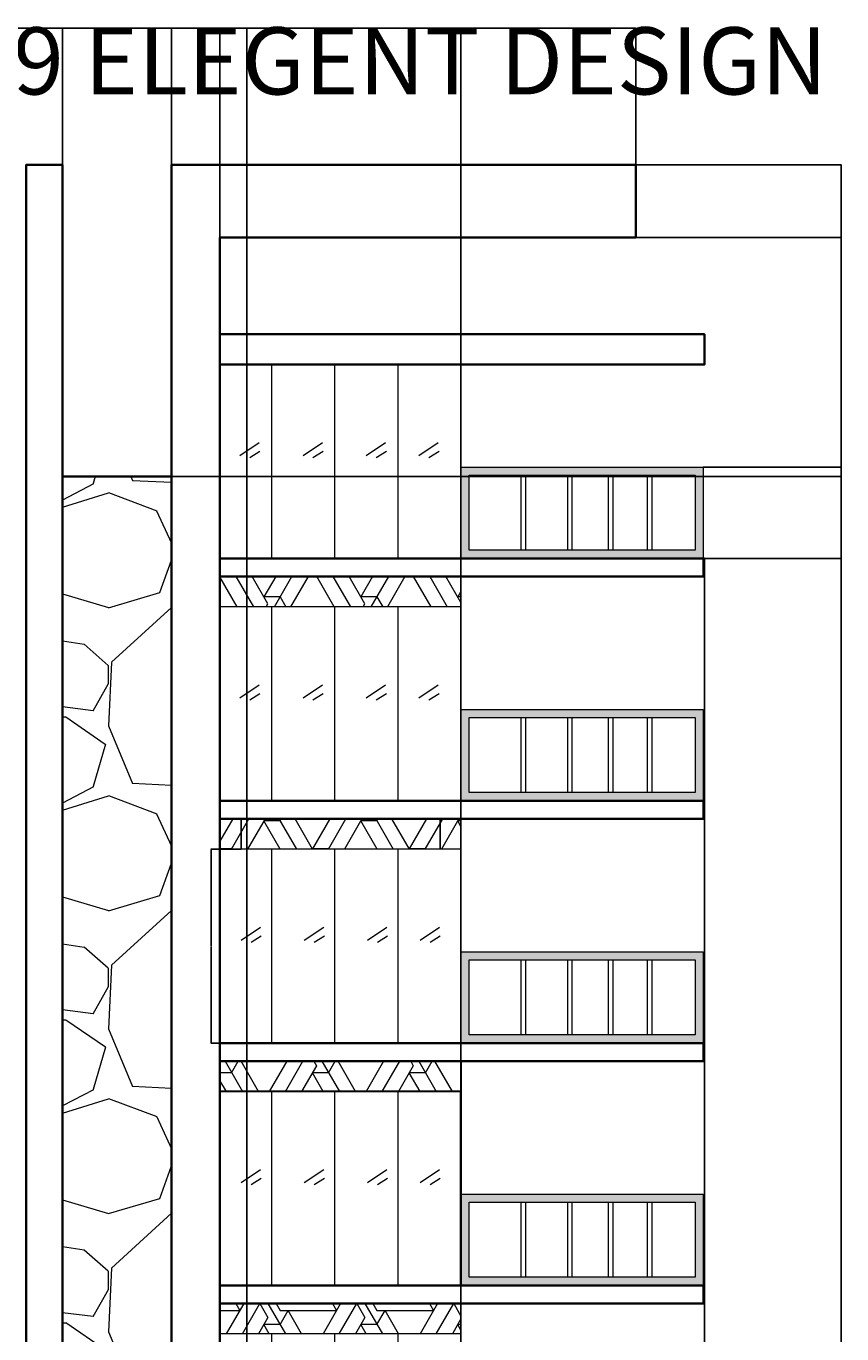
# Model space of a CAD drawing. Units: inches. Extents: x -38 to 698, y -57 to 1364.
# Tile 5 of 5: x 294 to 698, y 716 to 1364. Entities that reach past the tile are written whole.
import ezdxf

# ---------------------------------------------------------------- set-up
doc = ezdxf.new("R2010")
doc.units = ezdxf.units.IN
doc.header["$MEASUREMENT"] = 0
for name, color, linetype, lineweight in [('A-ANNO-DIMS', 2, 'Continuous', 18), ('A-ANNO-TEXT', 7, 'Continuous', 25), ('A-ELEV-PATT', 8, 'Continuous', 13), ('A-FLOR', 7, 'Continuous', 30), ('A-FLOR-HRAL', 7, 'Continuous', 20), ('A-GLAZ', 4, 'Continuous', 18), ('A-ROOF', 7, 'Continuous', 35), ('A-WALL', 7, 'Continuous', 35), ('A-WALL-PATT', 8, 'Continuous', 13)]:
    doc.layers.add(name, color=color, linetype=linetype, lineweight=lineweight)
doc.styles.get("Standard").update_dxf_attribs({"font": 'arial.ttf'})
doc.dimstyles.get("Standard").update_dxf_attribs({"dimtxt": 0.18, "dimasz": 0.18, "dimexe": 0.18, "dimexo": 0.0625, "dimgap": 0.09, "dimtad": 0, "dimtih": 1, "dimtoh": 1, "dimdec": 4, "dimzin": 0, "dimdsep": 46, "dimtxsty": 'Standard', "dimcen": 0.09, "dimadec": 0, "dimazin": 0, "dimtfac": 1, "dimtdec": 4, "dimtofl": 0, "dimtmove": 0, "dimatfit": 3, "dimfxl": 1, "dimtolj": 1, "dimtzin": 0, "dimarcsym": 0})

# ---------------------------------------------------------------- blocks, each defined once
blk = doc.blocks.new('WINDOW-4L-RH')
for p, q in [((15.6, 96), (15.6, 0)), ((46.9, 96), (46.9, 0)), ((78.2, 96), (78.2, 0)), ((0, 50.99), (9.6, 57.46)), ((4.92, 50.03), (9.96, 53.14)), ((31.3, 50.99), (40.9, 57.46)), ((36.22, 50.03), (41.26, 53.14)), ((62.61, 50.99), (72.2, 57.46)), ((67.52, 50.03), (72.56, 53.14)), ((88.7, 50.99), (98.29, 57.46)), ((93.62, 50.03), (98.65, 53.14))]:
    blk.add_line(p, q)
blk = doc.blocks.new('WINDOW-4L-RH-ALT')
for p, q in [((14.97, 96), (14.97, 0)), ((46.28, 96), (46.28, 0)), ((77.58, 96), (77.58, 0)), ((0, 50.99), (9.6, 57.46)), ((4.92, 50.03), (9.96, 53.14)), ((31.3, 50.99), (40.9, 57.46)), ((36.22, 50.03), (41.26, 53.14)), ((62.61, 50.99), (72.2, 57.46)), ((67.52, 50.03), (72.56, 53.14)), ((88.7, 50.99), (98.29, 57.46)), ((93.61, 50.03), (98.65, 53.14))]:
    blk.add_line(p, q)
blk = doc.blocks.new('BALCONY-GUARD-PICKETS')
for p, q in [((0, 37.13), (0, 0)), ((2.41, 0), (2.41, 37.13)), ((19.25, 37.13), (19.25, 0)), ((21.65, 0), (21.65, 37.13)), ((39.53, 37.13), (39.53, 0)), ((41.93, 0), (41.93, 37.13)), ((62.55, 37.13), (62.55, 0)), ((64.96, 0), (64.96, 37.13))]:
    blk.add_line(p, q)
blk = doc.blocks.new('*D14')
at = {"layer": 'A-ANNO-DIMS', "color": 0, "lineweight": -2, "transparency": 16777216}
for p, q in [((400.18, 956.28), (400.18, 971.19)), ((400.36, 971.01), (448.46, 971.01)), ((498.65, 971.01), (450.56, 971.01)), ((498.83, 956.28), (498.83, 971.19))]:
    blk.add_line(p, q, dxfattribs=at)
at = {"layer": 'A-ANNO-DIMS', "color": 0, "transparency": 16777216}
for points in [[(400.36, 971.04), (400.36, 970.98), (400.18, 971.01)], [(498.65, 971.04), (498.65, 970.98), (498.83, 971.01)]]:
    blk.add_solid(points, dxfattribs=at)
at = {"layer": 'Defpoints', "color": 0, "transparency": 16777216}
for p in [(498.83, 971.01), (400.18, 956.21), (498.83, 956.21)]:
    blk.add_point(p, dxfattribs=at)
at = {"layer": 'A-ANNO-DIMS', "color": 0, "transparency": 16777216, "insert": (449.51, 971.01), "char_height": 0.18, "attachment_point": 5}
blk.add_mtext('\\A1;ALT. RH 99 TYP.', dxfattribs=at)
blk = doc.blocks.new('*D15')
at = {"layer": 'A-ANNO-DIMS', "color": 0, "lineweight": -2, "transparency": 16777216}
for p, q in [((400.12, 956.21), (385.2, 956.21)), ((385.38, 956.03), (385.38, 908.4)), ((385.38, 860.39), (385.38, 908.03)), ((400.12, 860.21), (385.2, 860.21))]:
    blk.add_line(p, q, dxfattribs=at)
at = {"layer": 'A-ANNO-DIMS', "color": 0, "transparency": 16777216}
for points in [[(385.35, 956.03), (385.41, 956.03), (385.38, 956.21)], [(385.35, 860.39), (385.41, 860.39), (385.38, 860.21)]]:
    blk.add_solid(points, dxfattribs=at)
at = {"layer": 'Defpoints', "color": 0, "transparency": 16777216}
for p in [(385.38, 956.21), (400.18, 956.21), (400.18, 860.21)]:
    blk.add_point(p, dxfattribs=at)
at = {"layer": 'A-ANNO-DIMS', "color": 0, "transparency": 16777216, "insert": (385.38, 908.21), "char_height": 0.18, "attachment_point": 5}
blk.add_mtext('\\A1;96 TYP.', dxfattribs=at)
blk = doc.blocks.new('*D23')
at = {"layer": 'A-ANNO-DIMS', "color": 0, "lineweight": -2, "transparency": 16777216}
for p, q in [((595.72, 1295.04), (697.57, 1295.04)), ((697.39, 1294.86), (697.39, 653.31)), ((697.39, 11.39), (697.39, 652.94)), ((629.75, 11.21), (697.57, 11.21))]:
    blk.add_line(p, q, dxfattribs=at)
at = {"layer": 'A-ANNO-DIMS', "color": 0, "transparency": 16777216}
for points in [[(697.36, 1294.86), (697.42, 1294.86), (697.39, 1295.04)], [(697.36, 11.39), (697.42, 11.39), (697.39, 11.21)]]:
    blk.add_solid(points, dxfattribs=at)
at = {"layer": 'Defpoints', "color": 0, "transparency": 16777216}
for p in [(595.66, 1295.04), (697.39, 1295.04), (629.69, 11.21)]:
    blk.add_point(p, dxfattribs=at)
at = {"layer": 'A-ANNO-DIMS', "color": 0, "transparency": 16777216, "insert": (697.39, 653.13), "char_height": 0.18, "attachment_point": 5}
blk.add_mtext('\\A1;1283.8', dxfattribs=at)
blk = doc.blocks.new('*D25')
at = {"layer": 'A-ANNO-DIMS', "color": 0, "lineweight": -2, "transparency": 16777216}
for p, q in [((269.69, 1100.15), (269.69, -56.67)), ((389.69, 1100.15), (389.69, -56.67)), ((269.87, -56.49), (329.41, -56.49)), ((389.51, -56.49), (329.97, -56.49))]:
    blk.add_line(p, q, dxfattribs=at)
at = {"layer": 'A-ANNO-DIMS', "color": 0, "transparency": 16777216}
for points in [[(269.87, -56.46), (269.87, -56.52), (269.69, -56.49)], [(389.51, -56.46), (389.51, -56.52), (389.69, -56.49)]]:
    blk.add_solid(points, dxfattribs=at)
at = {"layer": 'Defpoints', "color": 0, "transparency": 16777216}
for p in [(269.69, 1100.21), (389.69, 1100.21), (389.69, -56.49)]:
    blk.add_point(p, dxfattribs=at)
at = {"layer": 'A-ANNO-DIMS', "color": 0, "transparency": 16777216, "insert": (329.69, -56.49), "char_height": 0.18, "attachment_point": 5}
blk.add_mtext('\\A1;120', dxfattribs=at)
blk = doc.blocks.new('*D26')
at = {"layer": 'A-ANNO-DIMS', "color": 0, "lineweight": -2, "transparency": 16777216}
for p, q in [((389.69, 1100.15), (389.69, -56.67)), ((629.69, 1100.15), (629.69, -56.67)), ((389.87, -56.49), (509.4, -56.49)), ((629.51, -56.49), (509.98, -56.49))]:
    blk.add_line(p, q, dxfattribs=at)
at = {"layer": 'A-ANNO-DIMS', "color": 0, "transparency": 16777216}
for points in [[(389.87, -56.46), (389.87, -56.52), (389.69, -56.49)], [(629.51, -56.46), (629.51, -56.52), (629.69, -56.49)]]:
    blk.add_solid(points, dxfattribs=at)
at = {"layer": 'Defpoints', "color": 0, "transparency": 16777216}
for p in [(389.69, 1100.21), (629.69, 1100.21), (629.69, -56.49)]:
    blk.add_point(p, dxfattribs=at)
at = {"layer": 'A-ANNO-DIMS', "color": 0, "transparency": 16777216, "insert": (509.69, -56.49), "char_height": 0.18, "attachment_point": 5}
blk.add_mtext('\\A1;240', dxfattribs=at)
blk = doc.blocks.new('*D28')
at = {"layer": 'A-ANNO-DIMS', "color": 0, "lineweight": -2, "transparency": 16777216}
for p, q in [((389.69, 380.28), (389.69, 1362.92)), ((389.87, 1362.74), (448.92, 1362.74)), ((508.88, 1362.74), (449.83, 1362.74)), ((509.06, 380.28), (509.06, 1362.92))]:
    blk.add_line(p, q, dxfattribs=at)
at = {"layer": 'A-ANNO-DIMS', "color": 0, "transparency": 16777216}
for points in [[(389.87, 1362.77), (389.87, 1362.71), (389.69, 1362.74)], [(508.88, 1362.77), (508.88, 1362.71), (509.06, 1362.74)]]:
    blk.add_solid(points, dxfattribs=at)
at = {"layer": 'Defpoints', "color": 0, "transparency": 16777216}
for p in [(509.06, 1362.74), (389.69, 380.21), (509.06, 380.21)]:
    blk.add_point(p, dxfattribs=at)
at = {"layer": 'A-ANNO-DIMS', "color": 0, "transparency": 16777216, "insert": (449.37, 1362.74), "char_height": 0.18, "attachment_point": 5}
blk.add_mtext('\\A1;119.38', dxfattribs=at)
blk = doc.blocks.new('*D44')
at = {"layer": 'A-ANNO-DIMS', "color": 0, "lineweight": -2, "transparency": 16777216}
for p, q in [((365.69, 1295.1), (365.69, 1362.92)), ((365.87, 1362.74), (480.21, 1362.74)), ((595.48, 1362.74), (481.14, 1362.74)), ((595.66, 1295.1), (595.66, 1362.92))]:
    blk.add_line(p, q, dxfattribs=at)
at = {"layer": 'A-ANNO-DIMS', "color": 0, "transparency": 16777216}
for points in [[(365.87, 1362.77), (365.87, 1362.71), (365.69, 1362.74)], [(595.48, 1362.77), (595.48, 1362.71), (595.66, 1362.74)]]:
    blk.add_solid(points, dxfattribs=at)
at = {"layer": 'Defpoints', "color": 0, "transparency": 16777216}
for p in [(595.66, 1362.74), (365.69, 1295.04), (595.66, 1295.04)]:
    blk.add_point(p, dxfattribs=at)
at = {"layer": 'A-ANNO-DIMS', "color": 0, "transparency": 16777216, "insert": (480.67, 1362.74), "char_height": 0.18, "attachment_point": 5}
blk.add_mtext('\\A1;229.97', dxfattribs=at)
blk = doc.blocks.new('*D46')
at = {"layer": 'A-ANNO-DIMS', "color": 0, "lineweight": -2, "transparency": 16777216}
for p, q in [((595.72, 1295.04), (697.57, 1295.04)), ((697.39, 1294.86), (697.39, 1277.22)), ((697.39, 1259.22), (697.39, 1276.85)), ((595.72, 1259.04), (697.57, 1259.04))]:
    blk.add_line(p, q, dxfattribs=at)
at = {"layer": 'A-ANNO-DIMS', "color": 0, "transparency": 16777216}
for points in [[(697.36, 1294.86), (697.42, 1294.86), (697.39, 1295.04)], [(697.36, 1259.22), (697.42, 1259.22), (697.39, 1259.04)]]:
    blk.add_solid(points, dxfattribs=at)
at = {"layer": 'Defpoints', "color": 0, "transparency": 16777216}
for p in [(595.66, 1295.04), (697.39, 1295.04), (595.66, 1259.04)]:
    blk.add_point(p, dxfattribs=at)
at = {"layer": 'A-ANNO-DIMS', "color": 0, "transparency": 16777216, "insert": (697.39, 1277.04), "char_height": 0.18, "attachment_point": 5}
blk.add_mtext('\\A1;36', dxfattribs=at)
blk = doc.blocks.new('*D48')
at = {"layer": 'A-ANNO-DIMS', "color": 0, "lineweight": -2, "transparency": 16777216}
for p, q in [((255.72, 101.28), (255.72, 1362.92)), ((255.9, 1362.74), (328.99, 1362.74)), ((402.85, 1362.74), (329.76, 1362.74)), ((403.03, 101.28), (403.03, 1362.92))]:
    blk.add_line(p, q, dxfattribs=at)
at = {"layer": 'A-ANNO-DIMS', "color": 0, "transparency": 16777216}
for points in [[(255.9, 1362.77), (255.9, 1362.71), (255.72, 1362.74)], [(402.85, 1362.77), (402.85, 1362.71), (403.03, 1362.74)]]:
    blk.add_solid(points, dxfattribs=at)
at = {"layer": 'Defpoints', "color": 0, "transparency": 16777216}
for p in [(403.03, 1362.74), (255.72, 101.21), (403.03, 101.21)]:
    blk.add_point(p, dxfattribs=at)
at = {"layer": 'A-ANNO-DIMS', "color": 0, "transparency": 16777216, "insert": (329.37, 1362.74), "char_height": 0.18, "attachment_point": 5}
blk.add_mtext('\\A1;147.3', dxfattribs=at)
blk = doc.blocks.new('*D49')
at = {"layer": 'A-ANNO-DIMS', "color": 0, "lineweight": -2, "transparency": 16777216}
for p, q in [((311.69, 1140.75), (311.69, 1362.92)), ((311.87, 1362.74), (338.47, 1362.74)), ((365.51, 1362.74), (338.9, 1362.74)), ((365.69, 1140.75), (365.69, 1362.92))]:
    blk.add_line(p, q, dxfattribs=at)
at = {"layer": 'A-ANNO-DIMS', "color": 0, "transparency": 16777216}
for points in [[(311.87, 1362.77), (311.87, 1362.71), (311.69, 1362.74)], [(365.51, 1362.77), (365.51, 1362.71), (365.69, 1362.74)]]:
    blk.add_solid(points, dxfattribs=at)
at = {"layer": 'Defpoints', "color": 0, "transparency": 16777216}
for p in [(365.69, 1362.74), (311.69, 1140.69), (365.69, 1140.69)]:
    blk.add_point(p, dxfattribs=at)
at = {"layer": 'A-ANNO-DIMS', "color": 0, "transparency": 16777216, "insert": (338.69, 1362.74), "char_height": 0.18, "attachment_point": 5}
blk.add_mtext('\\A1;54', dxfattribs=at)
blk = doc.blocks.new('*D50')
at = {"layer": 'A-ANNO-DIMS', "color": 0, "lineweight": -2, "transparency": 16777216}
for p, q in [((365.75, 1295.04), (697.57, 1295.04)), ((697.39, 1294.86), (697.39, 1218.05)), ((697.39, 1140.87), (697.39, 1217.68)), ((365.75, 1140.69), (697.57, 1140.69))]:
    blk.add_line(p, q, dxfattribs=at)
at = {"layer": 'A-ANNO-DIMS', "color": 0, "transparency": 16777216}
for points in [[(697.36, 1294.86), (697.42, 1294.86), (697.39, 1295.04)], [(697.36, 1140.87), (697.42, 1140.87), (697.39, 1140.69)]]:
    blk.add_solid(points, dxfattribs=at)
at = {"layer": 'Defpoints', "color": 0, "transparency": 16777216}
for p in [(365.69, 1295.04), (697.39, 1295.04), (365.69, 1140.69)]:
    blk.add_point(p, dxfattribs=at)
at = {"layer": 'A-ANNO-DIMS', "color": 0, "transparency": 16777216, "insert": (697.39, 1217.86), "char_height": 0.18, "attachment_point": 5}
blk.add_mtext('\\A1;154.34', dxfattribs=at)
blk = doc.blocks.new('*D51')
at = {"layer": 'A-ANNO-DIMS', "color": 0, "lineweight": -2, "transparency": 16777216}
for p, q in [((365.69, 1294.97), (365.69, -56.67)), ((389.69, 1258.97), (389.69, -56.67)), ((365.87, -56.49), (377.47, -56.49)), ((389.51, -56.49), (377.91, -56.49))]:
    blk.add_line(p, q, dxfattribs=at)
at = {"layer": 'A-ANNO-DIMS', "color": 0, "transparency": 16777216}
for points in [[(365.87, -56.46), (365.87, -56.52), (365.69, -56.49)], [(389.51, -56.46), (389.51, -56.52), (389.69, -56.49)]]:
    blk.add_solid(points, dxfattribs=at)
at = {"layer": 'Defpoints', "color": 0, "transparency": 16777216}
for p in [(365.69, 1295.04), (389.69, 1259.04), (389.69, -56.49)]:
    blk.add_point(p, dxfattribs=at)
at = {"layer": 'A-ANNO-DIMS', "color": 0, "transparency": 16777216, "insert": (377.69, -56.49), "char_height": 0.18, "attachment_point": 5}
blk.add_mtext('\\A1;24', dxfattribs=at)
blk = doc.blocks.new('*D54')
at = {"layer": 'A-ANNO-DIMS', "color": 0, "lineweight": -2, "transparency": 16777216}
for p, q in [((629.13, 1145.34), (697.57, 1145.34)), ((697.39, 1145.16), (697.39, 1122.96)), ((697.39, 1100.39), (697.39, 1122.6)), ((629.13, 1100.21), (697.57, 1100.21))]:
    blk.add_line(p, q, dxfattribs=at)
at = {"layer": 'A-ANNO-DIMS', "color": 0, "transparency": 16777216}
for points in [[(697.36, 1145.16), (697.42, 1145.16), (697.39, 1145.34)], [(697.36, 1100.39), (697.42, 1100.39), (697.39, 1100.21)]]:
    blk.add_solid(points, dxfattribs=at)
at = {"layer": 'Defpoints', "color": 0, "transparency": 16777216}
for p in [(629.06, 1145.34), (697.39, 1145.34), (629.06, 1100.21)]:
    blk.add_point(p, dxfattribs=at)
at = {"layer": 'A-ANNO-DIMS', "color": 0, "transparency": 16777216, "insert": (697.39, 1122.78), "char_height": 0.18, "attachment_point": 5}
blk.add_mtext('\\A1;45.13', dxfattribs=at)

msp = doc.modelspace()

# ---------------------------------------------------------------- hatches: boundary and pattern name
at = {"layer": 'A-ELEV-PATT', "transparency": 33554562}
h = msp.add_hatch(dxfattribs=at)
h.set_pattern_fill('HONEY', color=256, scale=40)
h.set_pattern_definition([(0, (-116.5534, -96.733), (7.5, 4.330127), [5, -10]), (120, (-116.5534, -96.733), (-7.5, 4.330127), [5, -10]), (60, (-116.5534, -96.733), (2e-15, 8.660254), [-10, 5])])
h.paths.add_polyline_path([(629.0638, 1145.3406), (509.0638, 1145.3406), (509.0638, 1100.2149), (629.0638, 1100.2149)])
h.paths.add_polyline_path([(625.0638, 1141.3406), (625.0638, 1104.2149), (513.0638, 1104.2149), (513.0638, 1141.3406)], flags=16)
h.paths.add_polyline_path([(629.0638, 1025.3406), (509.0638, 1025.3406), (509.0638, 980.2149), (629.0638, 980.2149)])
h.paths.add_polyline_path([(625.0638, 1021.3406), (625.0638, 984.2149), (513.0638, 984.2149), (513.0638, 1021.3406)], flags=16)
h.paths.add_polyline_path([(629.0638, 905.3406), (509.0638, 905.3406), (509.0638, 860.2149), (629.0638, 860.2149)])
h.paths.add_polyline_path([(625.0638, 901.3406), (625.0638, 864.2149), (513.0638, 864.2149), (513.0638, 901.3406)], flags=16)
h.paths.add_polyline_path([(629.0638, 785.3406), (509.0638, 785.3406), (509.0638, 740.2149), (629.0638, 740.2149)])
h.paths.add_polyline_path([(625.0638, 781.3406), (625.0638, 744.2149), (513.0638, 744.2149), (513.0638, 781.3406)], flags=16)
h.paths.add_polyline_path([(629.0638, 665.3406), (509.0638, 665.3406), (509.0638, 620.2149), (629.0638, 620.2149)])
h.paths.add_polyline_path([(625.0638, 661.3406), (625.0638, 624.2149), (513.0638, 624.2149), (513.0638, 661.3406)], flags=16)
h.paths.add_polyline_path([(629.0638, 545.3406), (509.0638, 545.3406), (509.0638, 500.2149), (629.0638, 500.2149)])
h.paths.add_polyline_path([(625.0638, 541.3406), (625.0638, 504.2149), (513.0638, 504.2149), (513.0638, 541.3406)], flags=16)
h.paths.add_polyline_path([(629.0638, 425.3406), (509.0638, 425.3406), (509.0638, 380.2149), (629.0638, 380.2149)])
h.paths.add_polyline_path([(625.0638, 421.3406), (625.0638, 384.2149), (513.0638, 384.2149), (513.0638, 421.3406)], flags=16)
h.paths.add_polyline_path([(629.0638, 296.3406), (509.0638, 296.3406), (509.0638, 251.2149), (629.0638, 251.2149)])
h.paths.add_polyline_path([(625.0638, 292.3406), (625.0638, 255.2149), (513.0638, 255.2149), (513.0638, 292.3406)], flags=16)
h.paths.add_polyline_path([(149.6854, 296.3406), (29.6854, 296.3406), (29.6854, 251.2149), (149.6854, 251.2149)])
h.paths.add_polyline_path([(145.6854, 292.3406), (145.6854, 255.2149), (33.6854, 255.2149), (33.6854, 292.3406)], flags=16)
h.paths.add_polyline_path([(149.6854, 425.3406), (29.6854, 425.3406), (29.6854, 380.2149), (149.6854, 380.2149)])
h.paths.add_polyline_path([(145.6854, 421.3406), (145.6854, 384.2149), (33.6854, 384.2149), (33.6854, 421.3406)], flags=16)
h.paths.add_polyline_path([(149.6854, 545.3406), (29.6854, 545.3406), (29.6854, 500.2149), (149.6854, 500.2149)])
h.paths.add_polyline_path([(33.6854, 504.2149), (33.6854, 541.3406), (145.6854, 541.3406), (145.6854, 504.2149)], flags=16)
h.paths.add_polyline_path([(149.6854, 665.3406), (29.6854, 665.3406), (29.6854, 620.2149), (149.6854, 620.2149)])
h.paths.add_polyline_path([(33.6854, 624.2149), (33.6854, 661.3406), (145.6854, 661.3406), (145.6854, 624.2149)], flags=16)
h.paths.add_polyline_path([(149.6854, 785.3406), (29.6854, 785.3406), (29.6854, 740.2149), (149.6854, 740.2149)])
h.paths.add_polyline_path([(33.6854, 744.2149), (33.6854, 781.3406), (145.6854, 781.3406), (145.6854, 744.2149)], flags=16)
h.paths.add_polyline_path([(149.6854, 905.3406), (29.6854, 905.3406), (29.6854, 860.2149), (149.6854, 860.2149)])
h.paths.add_polyline_path([(145.6854, 901.3406), (145.6854, 864.2149), (33.6854, 864.2149), (33.6854, 901.3406)], flags=16)
h.paths.add_polyline_path([(149.6854, 1025.3406), (29.6854, 1025.3406), (29.6854, 980.2149), (149.6854, 980.2149)])
h.paths.add_polyline_path([(33.6854, 984.2149), (33.6854, 1021.3406), (145.6854, 1021.3406), (145.6854, 984.2149)], flags=16)
h.paths.add_polyline_path([(149.6854, 1145.3406), (29.6854, 1145.3406), (29.6854, 1100.2149), (149.6854, 1100.2149)])
h.paths.add_polyline_path([(33.6854, 1104.2149), (33.6854, 1141.3406), (145.6854, 1141.3406), (145.6854, 1104.2149)], flags=16)
at = {"layer": 'A-WALL-PATT', "transparency": 33554625}
h = msp.add_hatch(dxfattribs=at)
h.set_pattern_fill('GRAVEL', color=256, scale=150)
h.set_pattern_definition([(228.0128, (-8.553, 53.267), (-1200, -1350), [20.1804, -1997.863]), (184.96974, (-22.0534, 38.267), (1800, 150), [34.63, -3428.3887]), (132.51045, (-56.553, 35.267), (1500, -1650), [24.418, -2417.405]), (267.2737, (-115.0534, -2.233), (150, 3000), [31.5357, -3122.0337]), (292.83365, (-116.5534, -33.733), (-750, 1800), [30.923, -3061.406]), (357.2737, (-104.5534, -62.233), (-3000, 150), [31.5357, -3122.0337]), (37.69424, (-73.0534, -63.733), (-1950, -1500), [41.7043, -4128.7273]), (72.25533, (-40.0534, -38.233), (1050, 3300), [39.373, -3897.9482]), (121.42957, (-28.0534, -0.733), (-1200, 1950), [31.6425, -3132.611]), (175.2364, (-44.553, 26.267), (1650, -150), [36.125, -1770.1144]), (222.39744, (-80.5534, 29.267), (-1800, -1650), [46.7172, -4625.0063]), (138.8141, (33.447, -3.733), (-1050, 900), [15.945, -1578.577]), (171.4692, (21.447, 6.767), (1950, -300), [30.3356, -3003.2267]), (225, (-8.55, 11.27), (-2e-14, -150), [21.213, -190.919]), (203.1986, (-19.053, 29.267), (750, 300), [11.424, -1130.942]), (291.8014, (-29.553, 24.767), (-150, 450), [16.155, -791.619]), (30.9638, (-23.553, 9.767), (450, 300), [26.239, -848.403]), (161.565, (-1.053, 23.267), (300, -150), [18.974, -455.368]), (16.38954, (-116.553, 24.767), (1500, 450), [26.58, -2631.427]), (70.3462, (-91.053, 32.267), (-600, -1650), [22.299, -2207.611]), (293.1986, (-1.053, 53.267), (-300, 750), [22.847, -1119.519]), (343.6105, (7.947, 32.267), (-1500, 450), [26.58, -2631.427]), (339.444, (-116.553, -68.233), (-750, 300), [25.632, -1255.9686]), (294.7751, (-92.553, -77.233), (-750, 1650), [21.477, -2126.1965]), (66.8014, (0.447, -96.733), (300, 750), [22.847, -1119.519]), (17.354, (9.447, -75.733), (-1950, -600), [25.1446, -2489.3135]), (69.444, (-73.053, -96.733), (-300, -750), [12.816, -1268.7846]), (101.31, (-8.553, -96.733), (-150, 600), [7.649, -757.204]), (165.9638, (-10.053, -89.233), (450, -150), [30.923, -587.543]), (186.009, (-40.053, -81.733), (1500, 150), [28.6575, -2837.0885]), (303.69, (-23.553, -3.733), (-150, 300), [21.633, -519.2]), (353.1572, (-11.5534, -21.733), (2550, -300), [37.769, -3739.1344]), (60.9454, (25.947, -26.233), (-600, -1050), [15.443, -1528.901]), (90, (33.45, -12.73), (-150, 150), [9, -141]), (120.2564, (-43.053, -77.233), (600, -1050), [20.8386, -2063.028]), (48.0128, (-53.553, -59.233), (1200, 1350), [40.361, -1977.683]), (0, (-26.55, -29.23), (150, 150), [39, -111]), (325.30485, (12.447, -29.233), (1500, -1050), [23.717, -2347.991]), (254.0546, (31.947, -42.733), (-150, -600), [21.84, -1070.176]), (207.646, (25.9466, -63.733), (-2850, -1500), [35.5598, -3520.421]), (175.4261, (-5.5534, -80.233), (-1950, 150), [37.62, -3724.361])])
h.paths.add_polyline_path([(311.6854, 107.2149), (365.6854, 107.2149), (365.6854, 851.2149), (365.6854, 971.2149), (365.6854, 1091.2149), (365.6854, 1140.6923), (311.6854, 1140.6923), (311.6854, 971.2149), (311.6854, 851.2149)])
at = {"layer": 'A-WALL-PATT', "transparency": 33554562}
h = msp.add_hatch(dxfattribs=at)
h.set_pattern_fill('ESCHER', color=256, scale=40)
h.set_pattern_definition([(60, (-116.553, -96.733), (-48, -1e-08), [44, -4]), (180, (-116.553, -96.733), (24, -41.5692), [44, -4]), (300, (-116.553, -96.733), (48, -1e-08), [44, -4]), (60, (-112.553, -96.733), (-48, -1e-08), [8, -40]), (300, (-112.553, -96.733), (48, -1e-08), [8, -40]), (60, (-118.553, -93.27), (-48, -1e-08), [8, -40]), (180, (-118.553, -93.27), (24, -41.5692), [8, -40]), (300, (-118.553, -100.197), (48, -1e-08), [8, -40]), (180, (-118.553, -100.197), (24, -41.5692), [8, -40]), (60, (-132.553, -96.733), (-48, -1e-08), [8, -40]), (300, (-132.553, -96.733), (48, -1e-08), [8, -40]), (60, (-108.553, -110.59), (-48, -1e-08), [8, -40]), (180, (-108.553, -110.59), (24, -41.5692), [8, -40]), (300, (-108.553, -82.877), (48, -1e-08), [8, -40]), (180, (-108.553, -82.877), (24, -41.5692), [8, -40]), (0, (-108.553, -89.805), (-24, 41.5692), [28, -20]), (0, (-108.553, -103.66), (-24, 41.5692), [28, -20]), (120, (-114.553, -86.34), (-48, 1e-08), [28, -20]), (120, (-126.553, -93.27), (-48, 1e-08), [28, -20]), (240, (-126.553, -100.197), (24, -41.5692), [28, -20]), (240, (-114.553, -107.125), (24, -41.5692), [28, -20])])
h.paths.add_polyline_path([(269.6854, 371.2149), (149.6854, 371.2149), (149.6854, 347.2149), (269.6854, 347.2149)])
h.paths.add_polyline_path([(509.0638, 371.2149), (389.6854, 371.2149), (389.6854, 347.2149), (509.0638, 347.2149)])
h.paths.add_polyline_path([(269.6854, 491.2149), (149.6854, 491.2149), (149.6854, 476.2149), (269.6854, 476.2149)])
h.paths.add_polyline_path([(509.0638, 491.2149), (389.6854, 491.2149), (389.6854, 476.2149), (509.0638, 476.2149)])
h.paths.add_polyline_path([(509.0638, 611.2149), (389.6854, 611.2149), (389.6854, 596.2149), (509.0638, 596.2149)])
h.paths.add_polyline_path([(269.6854, 611.2149), (149.6854, 611.2149), (149.6854, 596.2149), (269.6854, 596.2149)])
h.paths.add_polyline_path([(269.6854, 731.2149), (149.6854, 731.2149), (149.6854, 716.2149), (269.6854, 716.2149)])
h.paths.add_polyline_path([(509.0638, 731.2149), (389.6854, 731.2149), (389.6854, 716.2149), (509.0638, 716.2149)])
h.paths.add_polyline_path([(509.0638, 851.2149), (389.6854, 851.2149), (389.6854, 836.2149), (509.0638, 836.2149)])
h.paths.add_polyline_path([(269.6854, 851.2149), (149.6854, 851.2149), (149.6854, 836.2149), (269.6854, 836.2149)])
h.paths.add_polyline_path([(269.6854, 971.2149), (149.6854, 971.2149), (149.6854, 956.2149), (269.6854, 956.2149)])
h.paths.add_polyline_path([(509.0638, 971.2149), (389.6854, 971.2149), (389.6854, 956.2149), (509.0638, 956.2149)])
h.paths.add_polyline_path([(509.0638, 1091.2149), (389.6854, 1091.2149), (389.6854, 1076.2149), (509.0638, 1076.2149)])
h.paths.add_polyline_path([(269.6854, 1091.2149), (149.6854, 1091.2149), (149.6854, 1076.2149), (269.6854, 1076.2149)])

# ---------------------------------------------------------------- linework, layer by layer
at = {"layer": 'A-FLOR'}
for points in [[(629.6854, 1091.2149), (389.6854, 1091.2149), (629.6854, 1091.2149), (629.6854, 1100.2149), (389.6854, 1100.2149)], [(629.0638, 1100.2149), (389.6854, 1100.2149), (629.0638, 1100.2149), (629.0638, 1091.2149), (389.6854, 1091.2149), (629.0638, 1091.2149)], [(629.6854, 971.2149), (389.6854, 971.2149), (629.6854, 971.2149), (629.6854, 980.2149), (389.6854, 980.2149)], [(629.0638, 980.2149), (389.6854, 980.2149), (629.0638, 980.2149), (629.0638, 971.2149), (389.6854, 971.2149), (629.0638, 971.2149)], [(629.6854, 851.2149), (629.6854, 860.2149), (389.6854, 860.2149)], [(629.0638, 860.2149), (389.6854, 860.2149), (629.0638, 860.2149), (629.0638, 851.2149), (389.6854, 851.2149), (629.6854, 851.2149), (389.6854, 851.2149), (509.0638, 851.2149), (509.0638, 740.2149), (509.0638, 836.2149), (389.6854, 836.2149)], [(629.6854, 731.2149), (389.6854, 731.2149), (629.6854, 731.2149), (629.6854, 740.2149), (389.6854, 740.2149)], [(629.0638, 740.2149), (389.6854, 740.2149), (629.0638, 740.2149), (629.0638, 731.2149), (389.6854, 731.2149), (629.0638, 731.2149)]]:
    msp.add_lwpolyline(points, dxfattribs=at)
at = {"layer": 'A-FLOR-HRAL'}
for points in [[(509.0638, 1145.3406), (629.0638, 1145.3406), (629.0638, 1100.2149), (509.0638, 1100.2149)], [(513.0638, 1141.3406), (625.0638, 1141.3406), (625.0638, 1104.2149), (513.0638, 1104.2149)], [(509.0638, 1025.3406), (629.0638, 1025.3406), (629.0638, 980.2149), (509.0638, 980.2149)], [(513.0638, 1021.3406), (625.0638, 1021.3406), (625.0638, 984.2149), (513.0638, 984.2149)], [(509.0638, 905.3406), (629.0638, 905.3406), (629.0638, 860.2149), (509.0638, 860.2149)], [(513.0638, 901.3406), (625.0638, 901.3406), (625.0638, 864.2149), (513.0638, 864.2149)], [(509.0638, 785.3406), (629.0638, 785.3406), (629.0638, 740.2149), (509.0638, 740.2149)], [(513.0638, 781.3406), (625.0638, 781.3406), (625.0638, 744.2149), (513.0638, 744.2149)]]:
    msp.add_lwpolyline(points, close=True, dxfattribs=at)
at = {"layer": 'A-GLAZ'}
for p, q in [((509.0638, 1076.2149), (389.6854, 1076.2149)), ((509.0638, 956.2149), (389.6854, 956.2149)), ((509.0638, 716.2149), (389.6854, 716.2149))]:
    msp.add_line(p, q, dxfattribs=at)
for points in [[(509.0638, 1196.2149), (509.0638, 1100.2149)], [(509.0638, 620.2149), (509.0638, 731.2149), (509.0638, 620.2149), (509.0638, 500.2149), (509.0638, 611.2149)]]:
    msp.add_lwpolyline(points, dxfattribs=at)
for points in [[(509.0638, 980.2149), (509.0638, 1091.2149)], [(509.0638, 860.2149), (509.0638, 971.2149)]]:
    msp.add_lwpolyline(points, close=True, dxfattribs=at)
at = {"layer": 'A-ROOF'}
msp.add_lwpolyline([(389.6854, 1196.2149), (509.0638, 1196.2149), (629.6854, 1196.2149), (629.6854, 1211.2149), (389.6854, 1211.2149), (509.6854, 1211.2149)], dxfattribs=at)
at = {"layer": 'A-WALL'}
msp.add_line((311.6854, 1140.6923), (365.6854, 1140.6923), dxfattribs=at)
for points in [[(29.6854, 131.2149), (269.6854, 131.2149), (29.6854, 131.2149), (29.6854, 107.2149), (389.6854, 107.2149), (389.6854, 851.2149), (389.6854, 971.2149), (389.6854, 1091.2149), (389.6854, 1259.0353), (595.6569, 1259.0353), (595.6569, 1295.0353), (365.6854, 1295.0353), (365.6854, 1211.2149), (365.6854, 1091.2149), (365.6854, 971.2149), (365.6854, 851.2149), (365.6854, 107.2149)], [(293.6854, 107.2149), (293.6854, 851.2149), (293.6854, 971.2149), (293.6854, 1295.0353), (311.6854, 1295.0353), (311.6854, 1211.2149), (311.6854, 971.2149), (311.6854, 851.2149), (311.6854, 107.2149)]]:
    msp.add_lwpolyline(points, dxfattribs=at)

# ---------------------------------------------------------------- block references
at = {"layer": 'A-FLOR-HRAL', "rotation": 180}
for p in [(603.7292, 1141.3405), (603.7292, 1021.3405), (603.7292, 901.3405), (603.7292, 781.3405)]:
    msp.add_blockref('BALCONY-GUARD-PICKETS', p, dxfattribs=at)
at = {"layer": 'A-GLAZ'}
for name, p in [('WINDOW-4L-RH', (399.558, 1100.215)), ('WINDOW-4L-RH', (399.558, 980.215)), ('WINDOW-4L-RH-ALT', (400.18, 860.215)), ('WINDOW-4L-RH-ALT', (400.18, 740.215)), ('WINDOW-4L-RH', (399.558, 620.215))]:
    msp.add_blockref(name, p, dxfattribs=at)

# ---------------------------------------------------------------- texts
at = {"layer": 'A-ANNO-TEXT'}
msp.add_text('ELEVATION G+9 ELEGENT DESIGN', height=33.216729, dxfattribs=at).set_placement((-17.7381, 1329.9565))

# ---------------------------------------------------------------- dimensions: what is measured, and where the dimension line sits
at = {"layer": 'A-ANNO-DIMS'}
for base, p1, p2, override, picture, middle in [((403.029, 1362.7353), (255.7202, 101.2149), (403.029, 101.2149), {"dimdec": 1, "dimlfac": 1, "dimrnd": 0, "dimzin": 0, "dimdsep": 46, "dimlunit": 2}, '*D48', (329.3746, 1362.7353)), ((365.6854, 1362.7353), (311.6854, 1140.6923), (365.6854, 1140.6923), {"dimdec": 0, "dimlfac": 1, "dimrnd": 0, "dimzin": 0, "dimdsep": 46, "dimlunit": 2}, '*D49', (338.6854, 1362.7353)), ((595.6569, 1362.7353), (365.6854, 1295.0353), (595.6569, 1295.0353), {"dimdec": 2, "dimlfac": 1, "dimrnd": 0, "dimzin": 0, "dimdsep": 46, "dimlunit": 2}, '*D44', (480.6712, 1362.7353)), ((509.0638, 1362.7353), (389.6854, 380.2149), (509.0638, 380.2149), {"dimdec": 2, "dimlfac": 1, "dimrnd": 0, "dimzin": 0, "dimdsep": 46, "dimlunit": 2}, '*D28', (449.3746, 1362.7353)), ((389.6854, -56.4851), (365.6854, 1295.0353), (389.6854, 1259.0353), {"dimdec": 0, "dimlfac": 1, "dimrnd": 0, "dimzin": 0, "dimdsep": 46, "dimlunit": 2}, '*D51', (377.6854, -56.4851)), ((389.6854, -56.4851), (269.6854, 1100.2149), (389.6854, 1100.2149), {"dimdec": 0, "dimlfac": 1, "dimrnd": 0, "dimzin": 0, "dimdsep": 46, "dimlunit": 2}, '*D25', (329.6854, -56.4851)), ((629.6854, -56.4851), (389.6854, 1100.2149), (629.6854, 1100.2149), {"dimdec": 0, "dimlfac": 1, "dimrnd": 0, "dimzin": 0, "dimdsep": 46, "dimlunit": 2}, '*D26', (509.6854, -56.4851))]:
    dim = msp.add_linear_dim(base=base, p1=p1, p2=p2, dimstyle='Standard', override=override, dxfattribs=at)
    dim.commit()
    dim.dimension.update_dxf_attribs({"geometry": picture, "text_midpoint": middle})
for base, p1, p2, override, picture, middle in [((697.3854, 1295.0353), (365.6854, 1140.6923), (365.6854, 1295.0353), {"dimdec": 2, "dimlfac": 1, "dimrnd": 0, "dimzin": 0, "dimdsep": 46, "dimlunit": 2}, '*D50', (697.3854, 1217.8638)), ((697.3854, 1295.0353), (629.6854, 11.2149), (595.6569, 1295.0353), {"dimdec": 1, "dimlfac": 1, "dimrnd": 0, "dimzin": 0, "dimdsep": 46, "dimlunit": 2}, '*D23', (697.3854, 653.1251)), ((697.3854, 1295.0353), (595.6569, 1259.0353), (595.6569, 1295.0353), {"dimdec": 0, "dimlfac": 1, "dimrnd": 0, "dimzin": 0, "dimdsep": 46, "dimlunit": 2}, '*D46', (697.3854, 1277.0353)), ((697.3854, 1145.3406), (629.0638, 1100.2149), (629.0638, 1145.3406), {"dimdec": 2, "dimlfac": 1, "dimrnd": 0, "dimzin": 0, "dimdsep": 46, "dimlunit": 2}, '*D54', (697.3854, 1122.7777))]:
    dim = msp.add_linear_dim(base=base, p1=p1, p2=p2, angle=90, dimstyle='Standard', override=override, dxfattribs=at)
    dim.commit()
    dim.dimension.update_dxf_attribs({"geometry": picture, "text_midpoint": middle})
dim = msp.add_linear_dim(base=(498.8334, 971.013), p1=(400.1796, 956.2149), p2=(498.8334, 956.2149), text='ALT. RH <> TYP.', dimstyle='Standard', override={"dimdec": 0, "dimlfac": 1, "dimrnd": 0, "dimzin": 0, "dimdsep": 46, "dimlunit": 2}, dxfattribs=at)
dim.commit()
dim.dimension.update_dxf_attribs({"geometry": '*D14', "text_midpoint": (449.5065, 971.013)})
dim = msp.add_linear_dim(base=(385.3816, 956.2149), p1=(400.1796, 860.2149), p2=(400.1796, 956.2149), angle=90, text='<> TYP.', dimstyle='Standard', override={"dimdec": 0, "dimlfac": 1, "dimrnd": 0, "dimzin": 0, "dimdsep": 46, "dimlunit": 2}, dxfattribs=at)
dim.commit()
dim.dimension.update_dxf_attribs({"geometry": '*D15', "text_midpoint": (385.3816, 908.2149)})

doc.saveas('drawing.dxf')
